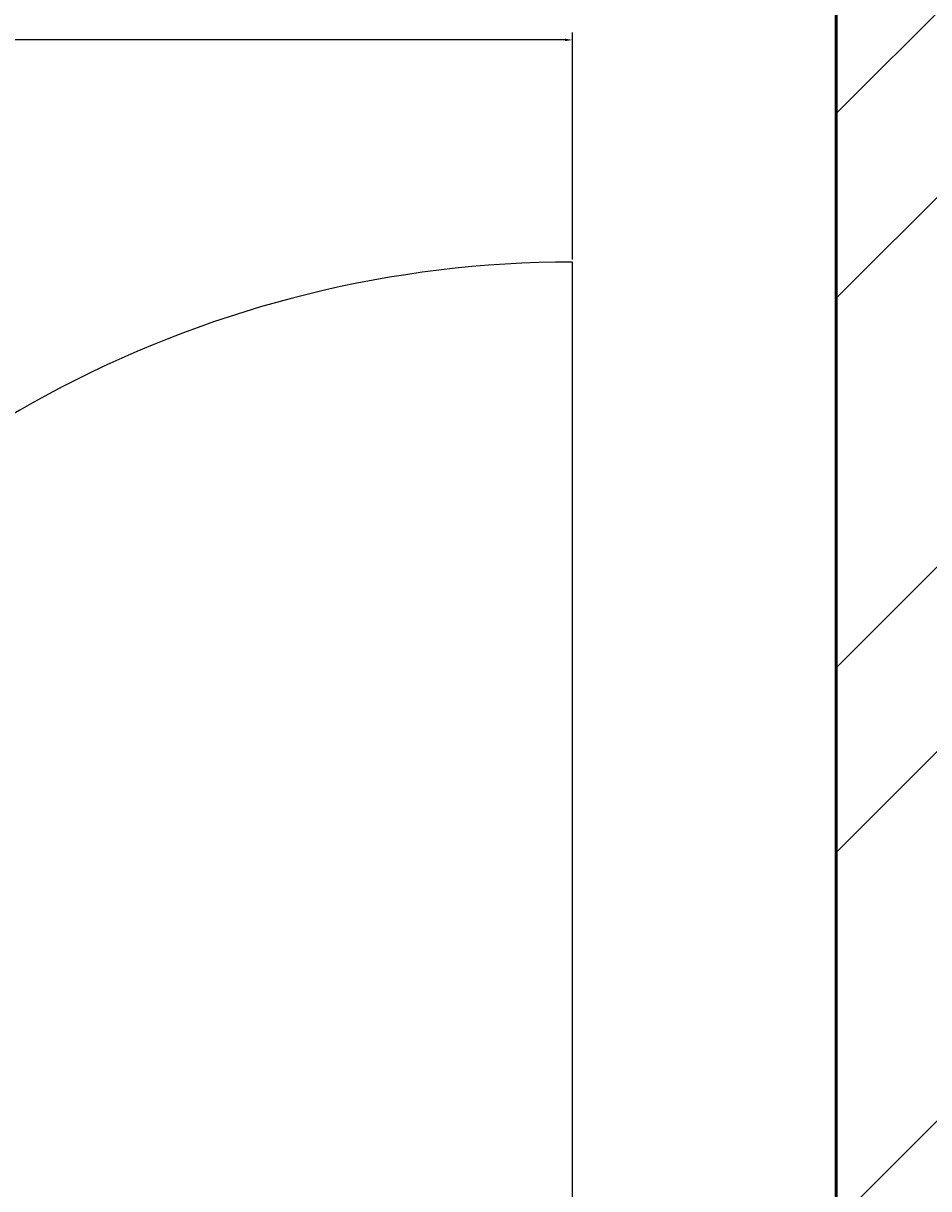
# Model space of a CAD drawing. Units: inches. Extents: x 1901 to 2863, y 888 to 2433.
# Tile 77 of 91: x 2586 to 2608, y 2094 to 2123. Entities that reach past the tile are written whole.
import ezdxf

# ---------------------------------------------------------------- set-up
doc = ezdxf.new("R2010")
doc.units = ezdxf.units.IN
for name, color, linetype, lineweight in [('A-ANNO-DIMS', 2, 'Continuous', 18), ('A-DOOR', 4, 'Continuous', 25), ('A-WALL', 7, 'Continuous', 50), ('A-WALL-PATT', 8, 'Continuous', 13)]:
    doc.layers.add(name, color=color, linetype=linetype, lineweight=lineweight)
doc.styles.get("Standard").update_dxf_attribs({"font": 'arial.ttf'})
doc.dimstyles.get("Standard").update_dxf_attribs({"dimtxt": 0.18, "dimasz": 0.18, "dimexe": 0.18, "dimexo": 0.0625, "dimgap": 0.09, "dimtad": 0, "dimtih": 1, "dimtoh": 1, "dimdec": 4, "dimzin": 0, "dimdsep": 46, "dimtxsty": 'Standard', "dimcen": 0.09, "dimadec": 0, "dimazin": 0, "dimtfac": 1, "dimtdec": 4, "dimtofl": 0, "dimtmove": 0, "dimatfit": 3, "dimfxl": 1, "dimtolj": 1, "dimtzin": 0, "dimarcsym": 0})

# ---------------------------------------------------------------- blocks, each defined once
blk = doc.blocks.new('DOOR-27')
blk.add_line((26.814, -0.016), (26.814, 35.984))
blk.add_arc((26.814, 9.122), 26.862, 90, 199.8893)
blk = doc.blocks.new('*D36')
at = {"layer": 'A-ANNO-DIMS', "color": 0, "lineweight": -2, "transparency": 16777216}
for p, q in [((2570.776, 2116.946), (2570.776, 2122.464)), ((2599.014, 2116.946), (2599.014, 2122.464)), ((2570.956, 2122.284), (2584.366, 2122.284)), ((2598.834, 2122.284), (2585.425, 2122.284))]:
    blk.add_line(p, q, dxfattribs=at)
at = {"layer": 'A-ANNO-DIMS', "color": 0, "transparency": 16777216}
for points in [[(2570.956, 2122.314), (2570.956, 2122.254), (2570.776, 2122.284)], [(2598.834, 2122.314), (2598.834, 2122.254), (2599.014, 2122.284)]]:
    blk.add_solid(points, dxfattribs=at)
at = {"layer": 'Defpoints', "color": 0, "transparency": 16777216}
for p in [(2599.014, 2122.284), (2570.776, 2116.884), (2599.014, 2116.884)]:
    blk.add_point(p, dxfattribs=at)
at = {"layer": 'A-ANNO-DIMS', "color": 0, "transparency": 16777216, "insert": (2584.895, 2122.284), "char_height": 0.18, "attachment_point": 5}
blk.add_mtext('\\A1;28 TYP.', dxfattribs=at)

msp = doc.modelspace()

# ---------------------------------------------------------------- hatches: boundary and pattern name
at = {"layer": 'A-WALL-PATT'}
h = msp.add_hatch(dxfattribs=at)
h.set_pattern_fill('ANSI32', color=256)
h.paths.add_polyline_path([(2192.501, 2274.134), (2141.264, 2274.134), (2141.264, 2269.634), (2192.501, 2269.634)])
h.paths.add_polyline_path([(2259.926, 2274.134), (2216.501, 2274.134), (2216.501, 2269.634), (2255.426, 2269.634), (2255.426, 2214.634), (2250.809, 2214.634), (2250.809, 2210.134), (2259.926, 2210.134), (2259.926, 2215.134), (2271.756, 2215.134), (2271.756, 2217.384), (2271.756, 2219.634), (2259.926, 2219.634)])
h.paths.add_polyline_path([(2171.426, 2269.634), (2166.926, 2269.634), (2166.926, 2219.634), (2121.238, 2219.634), (2121.238, 2215.134), (2166.926, 2215.134), (2166.926, 2083.134), (2161.807, 2083.134), (2161.807, 2078.634), (2171.426, 2078.634), (2176.996, 2078.634), (2176.996, 2080.884), (2176.996, 2083.134), (2171.426, 2083.134), (2171.426, 2210.134), (2230.912, 2210.134), (2230.912, 2212.384), (2230.912, 2214.634), (2171.426, 2214.634)])
h.paths.add_polyline_path([(2117.264, 2274.134), (2089.426, 2274.134), (2089.426, 2219.634), (2081.136, 2219.634), (2081.136, 2215.134), (2089.426, 2215.134), (2098.004, 2215.134), (2098.004, 2217.384), (2098.004, 2219.634), (2093.926, 2219.634), (2093.926, 2269.634), (2117.264, 2269.634), (2117.264, 2271.884)])
h.paths.add_polyline_path([(2343.426, 2219.634), (2329.295, 2219.634), (2329.295, 2215.134), (2338.926, 2215.134), (2338.926, 2184.739), (2343.426, 2184.739)])
h.paths.add_polyline_path([(2338.926, 2083.134), (2329.295, 2083.134), (2208.966, 2083.134), (2208.966, 2078.634), (2338.926, 2078.634)])
h.paths.add_polyline_path([(2343.426, 2136.739), (2338.926, 2136.739), (2338.926, 1872.634), (2343.426, 1872.634)])
h.paths.add_polyline_path([(2343.426, 1863.634), (2397.68, 1863.634), (2397.68, 1821.634), (2384.138, 1821.634), (2384.138, 1812.634), (2418.33, 1812.634), (2418.33, 1817.134), (2418.33, 1821.634), (2406.68, 1821.634), (2406.68, 1863.634), (2459.499, 1863.634), (2459.499, 1821.634), (2447.138, 1821.634), (2447.138, 1812.634), (2459.499, 1812.634), (2468.499, 1812.634), (2468.499, 1872.634), (2394.426, 1872.634), (2334.426, 1872.634), (2334.426, 1812.634), (2343.426, 1812.634), (2353.251, 1812.634), (2353.251, 1821.634), (2343.426, 1821.634)])
h.paths.add_polyline_path([(2510.014, 1872.634), (2468.499, 1872.634), (2468.499, 1868.134), (2510.014, 1868.134)])
h.paths.add_polyline_path([(2514.009, 1817.134), (2468.499, 1817.134), (2468.499, 1812.634), (2482.114, 1812.634), (2482.114, 1800.606), (2486.614, 1800.606), (2486.614, 1812.634), (2514.009, 1812.634)])
h.paths.add_polyline_path([(2299.247, 1814.884), (2299.247, 1817.134), (2295.926, 1817.134), (2295.926, 1854.169), (2293.676, 1854.169), (2291.426, 1854.169), (2291.426, 1817.134), (2266.109, 1817.134), (2266.109, 1812.634), (2299.247, 1812.634)])
h.paths.add_polyline_path([(2218.109, 1817.134), (2206.46, 1817.134), (2171.426, 1817.134), (2171.426, 1949.134), (2190.1, 1949.134), (2190.1, 1953.634), (2163.468, 1953.634), (2163.468, 1949.134), (2166.926, 1949.134), (2166.926, 1817.134), (2114.297, 1817.134), (2114.297, 1812.634), (2218.109, 1812.634)])
h.paths.add_polyline_path([(2029.426, 1970.922), (2024.926, 1970.922), (2024.926, 1912.717), (2029.426, 1912.717)])
h.paths.add_polyline_path([(2132.297, 1953.634), (2113.926, 1953.634), (2113.926, 1975.888), (2111.676, 1975.888), (2109.426, 1975.888), (2109.426, 1953.634), (2029.426, 1953.634), (2029.426, 1949.134), (2132.297, 1949.134)])
h.paths.add_polyline_path([(2029.426, 1853.606), (2029.31, 1853.606), (2029.31, 1853.606), (2029.426, 1853.606), (2029.426, 1864.717), (2024.926, 1864.717), (2024.926, 1812.634), (2066.297, 1812.634), (2066.297, 1814.884), (2066.297, 1817.134), (2029.426, 1817.134)])
h.paths.add_polyline_path([(2122.926, 2010.088), (2120.676, 2010.088), (2118.426, 2010.088), (2118.426, 2006.134), (2029.426, 2006.134), (2029.426, 2001.634), (2109.426, 2001.634), (2109.426, 1998.041), (2113.926, 1998.041), (2113.926, 2001.634), (2122.926, 2001.634)])
h.paths.add_polyline_path([(2029.426, 2031.376), (2024.926, 2031.376), (2024.926, 1994.922), (2027.176, 1994.922), (2029.426, 1994.922)])
h.paths.add_polyline_path([(2029.426, 2136.739), (2024.926, 2136.739), (2024.926, 2067.376), (2027.176, 2067.376), (2029.426, 2067.376)])
h.paths.add_polyline_path([(2125.618, 2083.134), (2029.426, 2083.134), (2029.426, 2078.634), (2118.426, 2078.634), (2118.426, 2030.715), (2122.926, 2030.715), (2122.926, 2078.634), (2125.618, 2078.634)])
h.paths.add_polyline_path([(2029.426, 2215.134), (2040.468, 2215.134), (2040.468, 2217.384), (2040.468, 2219.634), (2024.926, 2219.634), (2024.926, 2184.739), (2029.426, 2184.739), (2029.426, 2187.778)])
h.paths.add_polyline_path([(2686.426, 2274.134), (2659.284, 2274.134), (2659.284, 2269.634), (2681.926, 2269.634), (2681.926, 2219.634), (2676.816, 2219.634), (2676.816, 2215.134), (2681.926, 2215.134), (2697.011, 2215.134), (2697.011, 2217.384), (2697.011, 2219.634), (2686.426, 2219.634)])
h.paths.add_polyline_path([(2609.926, 2269.634), (2635.284, 2269.634), (2635.284, 2274.134), (2571.431, 2274.134), (2571.431, 2269.634), (2605.426, 2269.634), (2605.426, 2214.634), (2549.098, 2214.634), (2549.098, 2210.134), (2605.426, 2210.134), (2605.426, 2083.134), (2601.014, 2083.134), (2601.014, 2080.884), (2601.014, 2078.634), (2609.926, 2078.634), (2616.162, 2078.634), (2616.162, 2080.884), (2616.162, 2083.134), (2609.926, 2083.134), (2609.926, 2215.134), (2651.465, 2215.134), (2651.465, 2217.384), (2651.465, 2219.634), (2609.926, 2219.634)])
h.paths.add_polyline_path([(2521.426, 2269.634), (2547.431, 2269.634), (2547.431, 2271.884), (2547.431, 2274.134), (2516.926, 2274.134), (2516.926, 2219.634), (2506.41, 2219.634), (2506.41, 2215.134), (2516.926, 2215.134), (2516.926, 2210.134), (2525.402, 2210.134), (2525.402, 2212.384), (2525.402, 2214.634), (2521.426, 2214.634)])
h.paths.add_polyline_path([(2456.011, 2219.634), (2439.426, 2219.634), (2439.426, 2187.888), (2443.926, 2187.888), (2443.926, 2215.134), (2456.011, 2215.134)])
h.paths.add_polyline_path([(2752.926, 2219.634), (2739.485, 2219.634), (2739.485, 2215.134), (2748.426, 2215.134), (2748.426, 2187.888), (2752.926, 2187.888)])
h.paths.add_polyline_path([(2752.926, 2139.888), (2748.426, 2139.888), (2748.426, 2083.134), (2648.416, 2083.134), (2648.416, 2078.634), (2654.926, 2078.634), (2654.926, 2039.437), (2659.426, 2039.437), (2659.426, 2078.634), (2748.426, 2078.634), (2748.426, 2063.429), (2752.926, 2063.429)])
h.paths.add_polyline_path([(2752.926, 2010.634), (2659.426, 2010.634), (2659.426, 2015.652), (2654.926, 2015.652), (2654.926, 2010.634), (2605.426, 2010.634), (2605.426, 1920.967), (2609.926, 1920.967), (2609.926, 2006.134), (2748.426, 2006.134), (2748.426, 1982.466), (2752.926, 1982.466)])
h.paths.add_polyline_path([(2752.926, 2027.429), (2748.426, 2027.429), (2748.426, 2010.634), (2752.926, 2010.634)])
h.paths.add_polyline_path([(2748.426, 1886.134), (2609.926, 1886.134), (2609.926, 1889.719), (2605.426, 1889.719), (2605.426, 1861.262), (2609.926, 1861.262), (2609.926, 1881.634), (2748.426, 1881.634)])
h.paths.add_polyline_path([(2456.855, 2228.831), (2498.401, 2228.831), (2498.401, 2247.488), (2456.855, 2247.488)], flags=9)
h.paths.add_polyline_path([(2038.602, 2237.418), (2080.174, 2237.418), (2080.174, 2256.075), (2038.602, 2256.075)], flags=9)
h.paths.add_polyline_path([(2292.009, 1062.394), (2539.932, 1062.394), (2539.932, 1099.487), (2292.009, 1099.487)], flags=9)
h.paths.add_polyline_path([(2424.91, 1832.253), (2448.513, 1832.253), (2448.513, 1846.678), (2424.91, 1846.678)], flags=25)
h.paths.add_polyline_path([(2359.076, 1832.253), (2382.678, 1832.253), (2382.678, 1846.678), (2359.076, 1846.678)], flags=25)
h.paths.add_polyline_path([(2352.899, 1684.802), (2367.543, 1684.802), (2367.543, 1697.167), (2352.899, 1697.167)], flags=9)
h.paths.add_polyline_path([(2079.288, 1755.826), (2169.024, 1755.826), (2169.024, 1774.372), (2079.288, 1774.372)], flags=9)
h.paths.add_polyline_path([(2404.09, 1373.857), (2404.09, 1463.593), (2385.544, 1463.593), (2385.544, 1373.857)], flags=9)
h.paths.add_polyline_path([(2268.091, 2236.371), (2309.636, 2236.371), (2309.636, 2255.028), (2268.091, 2255.028)], flags=9)
h.paths.add_polyline_path([(2575.96, 1700.951), (2665.696, 1700.951), (2665.696, 1719.498), (2575.96, 1719.498)], flags=9)
h.paths.add_polyline_path([(2302.962, 1878.474), (2329.524, 1878.474), (2329.524, 1888.777), (2302.962, 1888.777)], flags=9)
h.paths.add_polyline_path([(2097.415, 2240.576), (2126.573, 2240.576), (2126.573, 2259.233), (2097.415, 2259.233)], flags=9)
h.paths.add_polyline_path([(2208.725, 2246.124), (2237.882, 2246.124), (2237.882, 2264.781), (2208.725, 2264.781)], flags=9)
h.paths.add_polyline_path([(2038.147, 1925.958), (2076.987, 1925.958), (2076.987, 1944.615), (2038.147, 1944.615)], flags=9)
h.paths.add_polyline_path([(2239.144, 1926.672), (2288.465, 1926.672), (2288.465, 1945.329), (2239.144, 1945.329)], flags=9)
h.paths.add_polyline_path([(2175.429, 2007.33), (2212.356, 2007.33), (2212.356, 2025.987), (2175.429, 2025.987)], flags=9)
h.paths.add_polyline_path([(2225.034, 2091.794), (2263.875, 2091.794), (2263.875, 2110.451), (2225.034, 2110.451)], flags=9)
h.paths.add_polyline_path([(2035.398, 2098.478), (2074.238, 2098.478), (2074.238, 2117.135), (2035.398, 2117.135)], flags=9)
h.paths.add_polyline_path([(2050.102, 2029.209), (2083.26, 2029.209), (2083.26, 2047.866), (2050.102, 2047.866)], flags=9)
h.paths.add_polyline_path([(2069.677, 1956.719), (2098.835, 1956.719), (2098.835, 1975.376), (2069.677, 1975.376)], flags=25)
h.paths.add_polyline_path([(2328.62, 1753.336), (2361.663, 1753.336), (2361.663, 1771.993), (2328.62, 1771.993)], flags=9)
h.paths.add_polyline_path([(2395.162, 2060.888), (2395.162, 2140.654), (2378.676, 2140.654), (2378.676, 2060.888)], flags=9)
h.paths.add_polyline_path([(2463.728, 2059.02), (2492.886, 2059.02), (2492.886, 2077.677), (2463.728, 2077.677)], flags=9)
h.paths.add_polyline_path([(2458.027, 2181.536), (2496.868, 2181.536), (2496.868, 2200.194), (2458.027, 2200.194)], flags=9)
h.paths.add_polyline_path([(2527.577, 2243.074), (2556.735, 2243.074), (2556.735, 2261.731), (2527.577, 2261.731)], flags=9)
h.paths.add_polyline_path([(2694.461, 2232.767), (2736.033, 2232.767), (2736.033, 2251.425), (2694.461, 2251.425)], flags=9)
h.paths.add_polyline_path([(2637.821, 2249.225), (2666.979, 2249.225), (2666.979, 2267.882), (2637.821, 2267.882)], flags=9)
h.paths.add_polyline_path([(2623.687, 2183.541), (2662.528, 2183.541), (2662.528, 2202.199), (2623.687, 2202.199)], flags=9)
h.paths.add_polyline_path([(2691.965, 2021.5), (2725.124, 2021.5), (2725.124, 2040.157), (2691.965, 2040.157)], flags=9)
h.paths.add_polyline_path([(2621.043, 1975.912), (2662.335, 1975.912), (2662.335, 1994.569), (2621.043, 1994.569)], flags=25)
h.paths.add_polyline_path([(2479.032, 1927.62), (2519.844, 1927.62), (2519.844, 1946.277), (2479.032, 1946.277)], flags=9)
h.paths.add_polyline_path([(2670.941, 1849.076), (2716.005, 1849.076), (2716.005, 1867.734), (2670.941, 1867.734)], flags=9)
h.paths.add_polyline_path([(2523.613, 1782.956), (2550.175, 1782.956), (2550.175, 1793.26), (2523.613, 1793.26)], flags=9)
h.paths.add_polyline_path([(2450.841, 1207.331), (2492.386, 1207.331), (2492.386, 1225.989), (2450.841, 1225.989)], flags=9)
h.paths.add_polyline_path([(2527.751, 1203.841), (2556.908, 1203.841), (2556.908, 1222.499), (2527.751, 1222.499)], flags=9)
h.paths.add_polyline_path([(2639.111, 1207.2), (2668.268, 1207.2), (2668.268, 1225.857), (2639.111, 1225.857)], flags=9)
h.paths.add_polyline_path([(2692.594, 1218.965), (2734.167, 1218.965), (2734.167, 1237.623), (2692.594, 1237.623)], flags=9)
h.paths.add_polyline_path([(2669.266, 1366.329), (2708.106, 1366.329), (2708.106, 1384.987), (2669.266, 1384.987)], flags=9)
h.paths.add_polyline_path([(2463.313, 1358.031), (2502.153, 1358.031), (2502.153, 1376.688), (2463.313, 1376.688)], flags=9)
h.paths.add_polyline_path([(2494.725, 1449.963), (2531.652, 1449.963), (2531.652, 1468.62), (2494.725, 1468.62)], flags=9)
h.paths.add_polyline_path([(2675.565, 1422.157), (2708.724, 1422.157), (2708.724, 1440.815), (2675.565, 1440.815)], flags=9)
h.paths.add_polyline_path([(2685.634, 1493.891), (2714.792, 1493.891), (2714.792, 1512.548), (2685.634, 1512.548)], flags=9)
h.paths.add_polyline_path([(2686.805, 1529.913), (2725.645, 1529.913), (2725.645, 1548.57), (2686.805, 1548.57)], flags=9)
h.paths.add_polyline_path([(2503.651, 1537.991), (2552.972, 1537.991), (2552.972, 1556.648), (2503.651, 1556.648)], flags=9)
h.paths.add_polyline_path([(2291.713, 1643.504), (2318.275, 1643.504), (2318.275, 1653.807), (2291.713, 1653.807)], flags=9)
h.paths.add_polyline_path([(2450.626, 1610.52), (2477.189, 1610.52), (2477.189, 1620.824), (2450.626, 1620.824)], flags=9)
h.paths.add_polyline_path([(2359.985, 1551.814), (2422.253, 1551.814), (2422.253, 1562.117), (2359.985, 1562.117)], flags=9)
h.paths.add_polyline_path([(2280.106, 1249.006), (2321.651, 1249.006), (2321.651, 1267.663), (2280.106, 1267.663)], flags=9)
h.paths.add_polyline_path([(2164.057, 1274.232), (2193.215, 1274.232), (2193.215, 1292.889), (2164.057, 1292.889)], flags=9)
h.paths.add_polyline_path([(2118.21, 1277.694), (2151.252, 1277.694), (2151.252, 1296.351), (2118.21, 1296.351)], flags=9)
h.paths.add_polyline_path([(2031.946, 1268.529), (2073.519, 1268.529), (2073.519, 1287.187), (2031.946, 1287.187)], flags=9)
h.paths.add_polyline_path([(2050.199, 1409.079), (2089.04, 1409.079), (2089.04, 1427.736), (2050.199, 1427.736)], flags=9)
h.paths.add_polyline_path([(2243.743, 1421.032), (2282.584, 1421.032), (2282.584, 1439.689), (2243.743, 1439.689)], flags=9)
h.paths.add_polyline_path([(2190.746, 1509.769), (2231.558, 1509.769), (2231.558, 1528.426), (2190.746, 1528.426)], flags=9)
h.paths.add_polyline_path([(2058.392, 1475.415), (2091.55, 1475.415), (2091.55, 1494.073), (2058.392, 1494.073)], flags=9)
h.paths.add_polyline_path([(2062.447, 1553.09), (2091.605, 1553.09), (2091.605, 1571.747), (2062.447, 1571.747)], flags=9)
h.paths.add_polyline_path([(2219.524, 1590.365), (2266.147, 1590.365), (2266.147, 1609.022), (2219.524, 1609.022)], flags=9)
h.paths.add_polyline_path([(2041.072, 1584.188), (2079.912, 1584.188), (2079.912, 1602.845), (2041.072, 1602.845)], flags=9)

# ---------------------------------------------------------------- linework, layer by layer
at = {"layer": 'A-WALL'}
msp.add_line((2605.426, 2210.134), (2605.426, 2083.134), dxfattribs=at)

# ---------------------------------------------------------------- block references
at = {"layer": 'A-DOOR'}
msp.add_blockref('DOOR-27', (2572.2, 2080.9), dxfattribs=at)

# ---------------------------------------------------------------- dimensions: what is measured, and where the dimension line sits
at = {"layer": 'A-ANNO-DIMS'}
dim = msp.add_linear_dim(base=(2599.014, 2122.284), p1=(2570.776, 2116.884), p2=(2599.014, 2116.884), text='<> TYP.', dimstyle='Standard', override={"dimdec": 0, "dimlfac": 1, "dimrnd": 0, "dimzin": 0, "dimdsep": 46, "dimlunit": 2}, dxfattribs=at)
dim.commit()
dim.dimension.update_dxf_attribs({"geometry": '*D36', "text_midpoint": (2584.895, 2122.284)})

doc.saveas('drawing.dxf')
